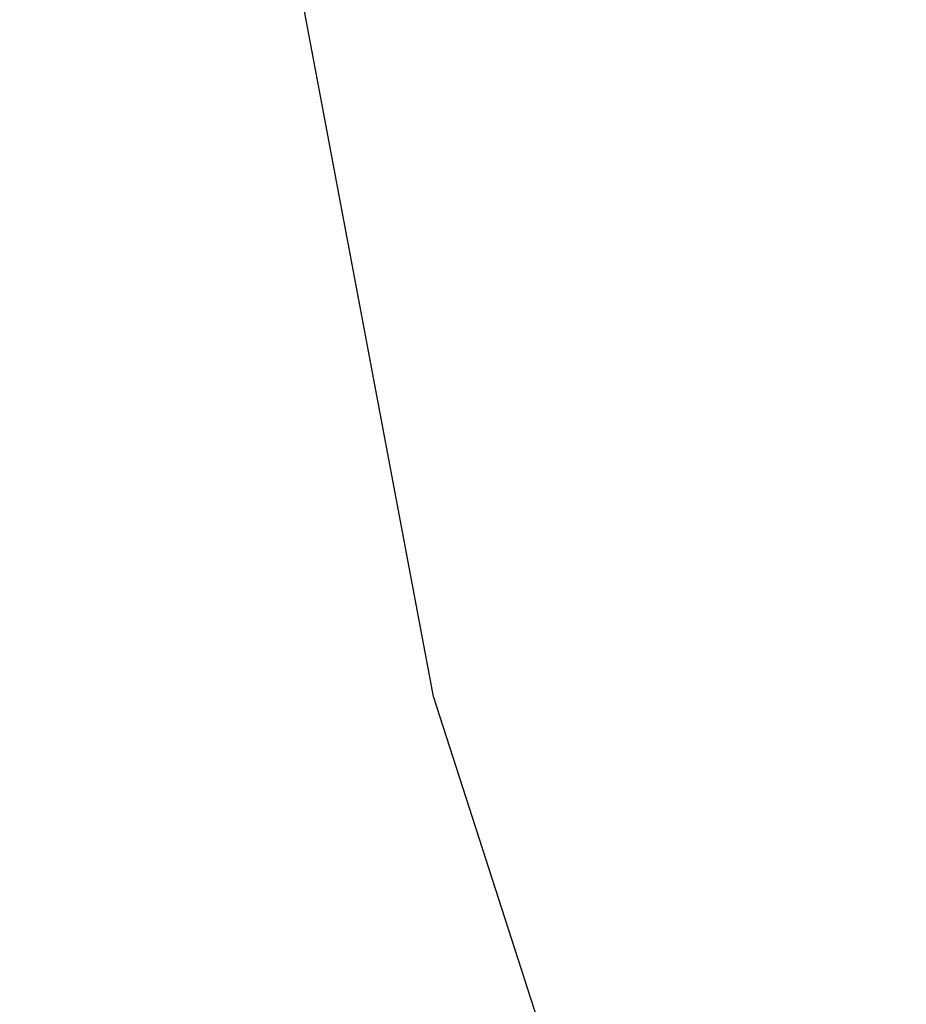
# Model space of a CAD drawing. Units: inches. Extents: x 3590 to 5167, y 65 to 1917.
# Tile 76 of 100: x 5045.839 to 5047.497, y 1787.19 to 1789.032. Entities that reach past the tile are written whole.
import ezdxf

# ---------------------------------------------------------------- set-up
doc = ezdxf.new("R2010")
doc.units = ezdxf.units.IN
for name, color, linetype, lineweight in [('A-ANNO-DIMS', 2, 'Continuous', 18), ('A-FLOR-PATT', 8, 'Continuous', 13), ('L-PLNT', 94, 'Continuous', 18)]:
    doc.layers.add(name, color=color, linetype=linetype, lineweight=lineweight)
doc.layers.add('DIENHOA', color=3, linetype='Continuous')
doc.styles.get("Standard").update_dxf_attribs({"font": 'arial.ttf'})
doc.dimstyles.new('ISO-25', dxfattribs={"dimtxt": 9, "dimasz": 2.5, "dimexe": 1.25, "dimexo": 0.625, "dimtad": 1, "dimdec": 1, "dimlunit": 3, "dimtxsty": 'Standard', "dimcen": 2.5, "dimadec": 0, "dimazin": 0, "dimtfac": 1, "dimtdec": 1, "dimtmove": 0, "dimatfit": 3, "dimfxl": 1, "dimarcsym": 0})

# ---------------------------------------------------------------- blocks, each defined once
blk = doc.blocks.new('Cay03_mb')
at = {"layer": 'DIENHOA'}
blk.add_lwpolyline([(23.687, -5.439), (-41, 82.202), (-91.832, 167.077), (-129.715, 249.451), (-155.553, 329.591), (-170.25, 407.762), (-174.71, 484.231), (-169.839, 559.263), (-156.54, 633.124)], dxfattribs=at)
blk = doc.blocks.new('*D322')
at = {"layer": 'A-ANNO-DIMS', "color": 0, "lineweight": -2, "transparency": 16777216}
for p, q in [((5035.7437, 1766.1842), (5035.7437, 1761.199)), ((5064.812, 1766.1842), (5064.812, 1761.199)), ((5038.2437, 1762.449), (5062.312, 1762.449)), ((5064.812, 1762.449), (5166.9911, 1762.449))]:
    blk.add_line(p, q, dxfattribs=at)
at = {"layer": 'A-ANNO-DIMS', "color": 0, "transparency": 16777216}
for points in [[(5038.2437, 1762.8657), (5038.2437, 1762.0323), (5035.7437, 1762.449)], [(5062.312, 1762.8657), (5062.312, 1762.0323), (5064.812, 1762.449)]]:
    blk.add_solid(points, dxfattribs=at)
at = {"layer": 'Defpoints', "color": 0, "transparency": 16777216}
for p in [(5035.7437, 1766.8092), (5064.812, 1766.8092), (5064.812, 1762.449)]:
    blk.add_point(p, dxfattribs=at)
at = {"layer": 'A-ANNO-DIMS', "color": 0, "transparency": 16777216, "insert": (5117.1516, 1767.6692), "char_height": 9, "attachment_point": 5}
blk.add_mtext('PLANT 2\'-5" TYP.', dxfattribs=at)

msp = doc.modelspace()

# ---------------------------------------------------------------- hatches: boundary and pattern name
at = {"layer": 'A-FLOR-PATT', "transparency": 33554687}
h = msp.add_hatch(dxfattribs=at)
h.set_pattern_fill('AR-HBONE', color=256, scale=0.2)
h.set_pattern_definition([(45, (-588.972, 0), (0, 28.73682), [60.96, -20.32]), (135, (-574.604, 14.368), (3e-15, 28.73682), [60.96, -20.32])])
h.paths.add_polyline_path([(5071.274, 1796.999), (4933.274, 1796.999), (4933.274, 1753.999), (4962.774, 1753.999, -0.414214), (4928.774, 1719.999), (4933.274, 1718.999), (4933.274, 1334.999), (5071.274, 1334.999)])
h.paths.add_polyline_path([(4951.78, 1521.0767), (4951.7151, 1521.0404), (4951.5634, 1520.8953)], flags=16)
h.paths.add_polyline_path([(4952.267, 1521.3764), (4952.1977, 1521.3711), (4952.1982, 1521.3556)], flags=0)
h.paths.add_polyline_path([(4967.0508, 1529.7283), (4965.2312, 1528.6944), (4963.4111, 1527.714), (4961.7565, 1526.8508), (4963.5889, 1527.4494), (4964.0356, 1527.478), (4962.9755, 1527.249), (4961.7602, 1526.852), (4959.7922, 1525.8341), (4958.005, 1524.8948), (4956.2403, 1523.9296), (4954.5039, 1522.9185), (4954.1294, 1522.6816), (4953.3605, 1521.9969), (4953.3656, 1521.9975), (4953.605, 1522.0637), (4955.1061, 1522.7608), (4956.9211, 1523.4341), (4958.6778, 1523.9151), (4960.3583, 1524.2004), (4961.9446, 1524.2861), (4964.1714, 1524.1085), (4965.9575, 1523.309), (4963.8627, 1522.9756), (4965.1874, 1522.499), (4963.3661, 1522.4971), (4961.5453, 1522.4868), (4959.7636, 1522.4608), (4958.3041, 1522.4188), (4957.9736, 1522.3883), (4956.3069, 1522.2324), (4954.7182, 1522.0714), (4953.2508, 1521.8992), (4953.5251, 1521.6228), (4954.3309, 1521.3788), (4956.2426, 1521.2299), (4958.0391, 1520.9295), (4959.6842, 1520.4834), (4961.1601, 1519.8957), (4963.107, 1518.8002), (4964.3929, 1517.3252), (4962.9731, 1517.726), (4964.5584, 1516.6606), (4965.4066, 1515.7078), (4963.5073, 1516.3218), (4961.68, 1517.0051), (4959.9348, 1517.7449), (4958.2821, 1518.5283), (4956.7322, 1519.3426), (4955.2953, 1520.1748), (4954.6715, 1520.5724), (4954.5128, 1520.6271), (4955.6585, 1519.3184), (4956.7026, 1517.9823), (4957.644, 1516.6466), (4958.4855, 1515.3344), (4959.55, 1513.524), (4960.4377, 1511.7694), (4958.8411, 1513.6196), (4957.4517, 1515.3249), (4955.8186, 1517.4586), (4956.6654, 1515.4476), (4957.1111, 1513.9229), (4957.4468, 1511.7143), (4957.0764, 1509.7929), (4956.5376, 1511.1103), (4955.9923, 1512.5689), (4955.4445, 1514.1251), (4954.8979, 1515.7352), (4954.3565, 1517.3555), (4953.8241, 1518.9425), (4953.3046, 1520.4525), (4953.0645, 1521.1156), (4952.9714, 1521.1461), (4952.9493, 1521.0865), (4952.7298, 1520.199), (4953.3698, 1518.0236), (4953.7571, 1516.3728), (4954.0512, 1514.7654), (4954.2645, 1513.2212), (4954.4712, 1511.1312), (4954.4971, 1510.4017), (4954.409, 1511.7601), (4954.2645, 1513.2212), (4954.0512, 1514.7654), (4953.7571, 1516.3728), (4953.3698, 1518.0236), (4952.8772, 1519.6981), (4952.7161, 1520.1412), (4952.533, 1519.0587), (4952.3743, 1517.7888), (4952.2192, 1516.3117), (4952.046, 1514.5999), (4951.8325, 1512.626), (4951.557, 1510.3626), (4951.2033, 1512.1682), (4950.8517, 1514.3393), (4950.9853, 1516.3759), (4951.6596, 1518.2862), (4952.5926, 1520.4808), (4952.3566, 1521.1299), (4951.855, 1520.3275), (4950.839, 1518.9083), (4949.7767, 1517.5866), (4948.9155, 1516.6173), (4948.111, 1515.2561), (4947.0891, 1513.5539), (4945.8894, 1511.6149), (4946.3259, 1513.4023), (4946.5624, 1514.2491), (4945.5277, 1513.3267), (4944.5811, 1512.5313), (4946.0177, 1514.5082), (4947.2044, 1516.0476), (4947.8933, 1517.3133), (4949.3069, 1518.7645), (4950.4142, 1519.7672), (4950.4513, 1519.8063), (4952.267, 1521.3764), (4951.6446, 1521.4932), (4950.4037, 1521.1795), (4948.0445, 1520.3587), (4946.1186, 1519.452), (4944.5718, 1518.4748), (4943.3496, 1517.4427), (4941.997, 1515.9197), (4941.6615, 1515.2748), (4942.8133, 1516.9897), (4944.5718, 1518.4748), (4946.1186, 1519.452), (4948.0445, 1520.3587), (4950.4037, 1521.1795), (4951.6446, 1521.4932), (4949.6468, 1521.8678), (4948.5998, 1521.7563), (4947.1263, 1521.5699), (4945.4202, 1521.3476), (4943.4497, 1521.1046), (4941.1832, 1520.856), (4942.8603, 1521.6126), (4943.8731, 1522.0301), (4942.9522, 1521.9093), (4941.4097, 1521.4851), (4939.5429, 1520.6702), (4938.9677, 1520.2255), (4940.7328, 1521.299), (4942.9522, 1521.9093), (4943.7018, 1522.0077), (4945.8942, 1522.7), (4947.5649, 1522.714), (4948.9209, 1522.5657), (4951.1314, 1522.1827), (4950.9706, 1522.2969), (4948.1292, 1523.0056), (4946.035, 1523.7067), (4944.2323, 1524.5214), (4942.7069, 1525.4611), (4941.4442, 1526.5371), (4940.4297, 1527.7606), (4939.6489, 1529.1431), (4941.4209, 1528.1223), (4943.1474, 1527.1325), (4944.8409, 1526.1746), (4946.5139, 1525.2496), (4948.1789, 1524.3586), (4948.3646, 1524.2634), (4946.4753, 1526.0446), (4945.1808, 1527.5404), (4944.1904, 1529.0334), (4943.4956, 1530.5398), (4943.2781, 1531.3597), (4942.4985, 1531.919), (4943.1135, 1531.7625), (4942.9593, 1533.6586), (4944.1395, 1531.9886), (4944.6117, 1531.3234), (4946.2016, 1530.4634), (4947.4857, 1529.5093), (4948.7903, 1528.2265), (4950.3675, 1526.2375), (4949.4855, 1528.1555), (4948.8513, 1530.1225), (4948.4905, 1532.0413), (4948.3811, 1533.9182), (4948.5006, 1535.7599), (4948.827, 1537.5728), (4949.418, 1535.5653), (4949.9568, 1533.5693), (4950.4641, 1531.5861), (4950.9606, 1529.6167), (4951.3911, 1527.9545), (4951.7235, 1530.6869), (4952.2011, 1532.5799), (4952.8891, 1534.3296), (4953.7703, 1535.9512), (4954.8273, 1537.46), (4954.5214, 1535.3897), (4954.2731, 1533.9368), (4955.58, 1535.6627), (4956.7476, 1536.7386), (4956.1585, 1534.7803), (4955.5892, 1532.8733), (4955.0434, 1531.0058), (4954.5249, 1529.1658), (4954.0377, 1527.3413), (4953.6383, 1525.733), (4953.6114, 1525.5856), (4953.3981, 1524.1657), (4953.3822, 1524.0089), (4954.0696, 1525.4756), (4954.9121, 1527.0217), (4956.1363, 1528.8935), (4957.8467, 1530.577), (4959.376, 1531.5401), (4958.256, 1530.104), (4957.1428, 1528.6629), (4956.0663, 1527.2431), (4955.0558, 1525.8705), (4954.141, 1524.5715), (4953.3516, 1523.372), (4953.3108, 1523.303), (4953.2725, 1522.9248), (4953.261, 1522.3821), (4954.1031, 1523.3727), (4954.63, 1524.2838), (4955.9615, 1526.3577), (4957.23, 1528.1297), (4958.4206, 1529.6086), (4960.0367, 1531.3679), (4961.3736, 1532.3752), (4962.1015, 1532.77), (4961.0699, 1531.0611), (4959.9873, 1529.4381), (4958.8685, 1527.908), (4958.1505, 1527.0074), (4959.8029, 1528.0031), (4961.5885, 1528.7926), (4963.3909, 1529.3278), (4965.2112, 1529.6321)], flags=16)
h.paths.add_polyline_path([(4962.9439, 1523.1819), (4961.1071, 1523.4219), (4960.3921, 1523.3616), (4962.3496, 1523.3306)], flags=0)
h.paths.add_polyline_path([(5049.5413, 1584.5509), (5049.4764, 1584.5146), (5049.3247, 1584.3695)], flags=16)
h.paths.add_polyline_path([(5050.0283, 1584.8506), (5049.959, 1584.8453), (5049.9595, 1584.8298)], flags=0)
h.paths.add_polyline_path([(5042.3331, 1581.949), (5043.8799, 1582.9262), (5045.8057, 1583.8329), (5048.165, 1584.6537), (5049.4058, 1584.9674), (5047.408, 1585.342), (5046.3611, 1585.2305), (5044.8876, 1585.0441), (5043.1814, 1584.8218), (5041.211, 1584.5788), (5038.9445, 1584.3301), (5040.6215, 1585.0868), (5041.6343, 1585.5043), (5040.7134, 1585.3835), (5039.1709, 1584.9593), (5037.3041, 1584.1444), (5036.729, 1583.6997), (5038.4941, 1584.7732), (5040.7134, 1585.3835), (5041.4631, 1585.4819), (5043.6555, 1586.1742), (5045.3261, 1586.1882), (5046.6821, 1586.0399), (5048.8927, 1585.6569), (5048.7319, 1585.7711), (5045.8905, 1586.4798), (5043.7962, 1587.1809), (5041.9936, 1587.9956), (5040.4682, 1588.9353), (5039.2055, 1590.0113), (5038.1909, 1591.2348), (5037.4102, 1592.6172), (5039.1822, 1591.5965), (5040.9087, 1590.6067), (5042.6022, 1589.6488), (5044.2752, 1588.7238), (5045.9402, 1587.8327), (5046.1258, 1587.7375), (5044.2366, 1589.5188), (5042.9421, 1591.0146), (5041.9517, 1592.5076), (5041.2569, 1594.014), (5041.0393, 1594.8339), (5040.2598, 1595.3932), (5040.8748, 1595.2367), (5040.7205, 1597.1328), (5041.9008, 1595.4628), (5042.373, 1594.7976), (5043.9629, 1593.9376), (5045.2469, 1592.9834), (5046.5515, 1591.7007), (5048.1288, 1589.7116), (5047.2467, 1591.6297), (5046.6125, 1593.5967), (5046.2518, 1595.5155), (5046.1423, 1597.3924), (5046.2619, 1599.2341), (5046.5883, 1601.047), (5047.1793, 1599.0394), (5047.7181, 1597.0435), (5048.2254, 1595.0603), (5048.7218, 1593.0909), (5049.1524, 1591.4287), (5049.4848, 1594.1611), (5049.9623, 1596.0541), (5050.6504, 1597.8038), (5051.5316, 1599.4254), (5052.5885, 1600.9341), (5052.2827, 1598.8638), (5052.0344, 1597.411), (5053.3413, 1599.1369), (5054.5088, 1600.2128), (5053.9198, 1598.2545), (5053.3504, 1596.3475), (5052.8046, 1594.48), (5052.2862, 1592.6399), (5051.799, 1590.8155), (5051.3996, 1589.2072), (5051.3727, 1589.0598), (5051.1593, 1587.6398), (5051.1435, 1587.4831), (5051.8308, 1588.9498), (5052.6734, 1590.4959), (5053.8975, 1592.3677), (5055.6079, 1594.0512), (5057.1373, 1595.0143), (5056.0172, 1593.5782), (5054.9041, 1592.1371), (5053.8275, 1590.7172), (5052.8171, 1589.3447), (5051.9023, 1588.0457), (5051.1129, 1586.8462), (5051.0721, 1586.7772), (5051.0338, 1586.399), (5051.0223, 1585.8563), (5051.8644, 1586.8469), (5052.3913, 1587.7579), (5053.7228, 1589.8318), (5054.9913, 1591.6039), (5056.1818, 1593.0828), (5057.798, 1594.8421), (5059.1349, 1595.8494), (5059.8628, 1596.2442), (5058.8312, 1594.5353), (5057.7486, 1592.9123), (5056.6298, 1591.3822), (5055.9117, 1590.4816), (5057.5642, 1591.4773), (5059.3498, 1592.2667), (5061.1521, 1592.802), (5062.9724, 1593.1062), (5064.812, 1593.2025), (5062.9925, 1592.1686), (5061.1724, 1591.1882), (5059.5178, 1590.325), (5061.3501, 1590.9236), (5061.7968, 1590.9522), (5060.7368, 1590.7232), (5059.5215, 1590.3262), (5057.5535, 1589.3082), (5055.7662, 1588.369), (5054.0016, 1587.4038), (5052.2652, 1586.3927), (5051.8907, 1586.1558), (5051.1218, 1585.4711), (5051.1268, 1585.4717), (5051.3663, 1585.5379), (5052.8673, 1586.235), (5054.6823, 1586.9082), (5056.4391, 1587.3893), (5058.1196, 1587.6745), (5059.7058, 1587.7602), (5061.9327, 1587.5827), (5063.7188, 1586.7832), (5061.624, 1586.4498), (5062.9487, 1585.9732), (5061.1274, 1585.9713), (5059.3065, 1585.961), (5057.5249, 1585.935), (5056.0654, 1585.893), (5055.7348, 1585.8625), (5054.0682, 1585.7066), (5052.4795, 1585.5456), (5051.012, 1585.3733), (5051.2864, 1585.097), (5052.0921, 1584.853), (5054.0039, 1584.7041), (5055.8004, 1584.4037), (5057.4455, 1583.9576), (5058.9213, 1583.3699), (5060.8683, 1582.2744), (5062.1541, 1580.7994), (5060.7343, 1581.2001), (5062.3197, 1580.1348), (5063.1679, 1579.182), (5061.2686, 1579.796), (5059.4412, 1580.4793), (5057.696, 1581.2191), (5056.0434, 1582.0025), (5054.4934, 1582.8168), (5053.0565, 1583.649), (5052.4328, 1584.0466), (5052.2741, 1584.1013), (5053.4197, 1582.7925), (5054.4639, 1581.4565), (5055.4053, 1580.1208), (5056.2467, 1578.8086), (5057.3112, 1576.9982), (5058.1989, 1575.2435), (5056.6023, 1577.0938), (5055.213, 1578.7991), (5053.5799, 1580.9327), (5054.4266, 1578.9218), (5054.8724, 1577.3971), (5055.2081, 1575.1885), (5054.8377, 1573.2671), (5054.2988, 1574.5845), (5053.7536, 1576.0431), (5053.2057, 1577.5993), (5052.6592, 1579.2094), (5052.1178, 1580.8297), (5051.5854, 1582.4167), (5051.0658, 1583.9267), (5050.8258, 1584.5898), (5050.7327, 1584.6203), (5050.7106, 1584.5606), (5050.4911, 1583.6732), (5051.1311, 1581.4978), (5051.5183, 1579.847), (5051.8125, 1578.2396), (5052.0257, 1576.6954), (5052.2325, 1574.6054), (5052.2584, 1573.8759), (5052.1703, 1575.2342), (5052.0257, 1576.6954), (5051.8125, 1578.2396), (5051.5183, 1579.847), (5051.1311, 1581.4978), (5050.6384, 1583.1723), (5050.4774, 1583.6154), (5050.2943, 1582.5329), (5050.1355, 1581.263), (5049.9805, 1579.7859), (5049.8072, 1578.074), (5049.5938, 1576.1002), (5049.3182, 1573.8368), (5048.9646, 1575.6424), (5048.6129, 1577.8135), (5048.7466, 1579.8501), (5049.4209, 1581.7604), (5050.3539, 1583.955), (5050.1179, 1584.6041), (5049.6163, 1583.8017), (5048.6003, 1582.3825), (5047.538, 1581.0608), (5046.6768, 1580.0915), (5045.8722, 1578.7303), (5044.8504, 1577.0281), (5043.6506, 1575.0891), (5044.0871, 1576.8765), (5044.3237, 1577.7233), (5043.289, 1576.8009), (5042.3423, 1576.0054), (5043.779, 1577.9824), (5044.9657, 1579.5218), (5045.6546, 1580.7875), (5047.0681, 1582.2386), (5048.1754, 1583.2413), (5048.2126, 1583.2805), (5050.0283, 1584.8506), (5049.4058, 1584.9674), (5048.165, 1584.6537), (5045.8057, 1583.8329), (5043.8799, 1582.9262), (5042.3331, 1581.949), (5041.1109, 1580.9168), (5039.7582, 1579.3939), (5039.4227, 1578.7489), (5040.5746, 1580.4639)], flags=16)
h.paths.add_polyline_path([(4954.7987, 1533.1203), (4954.2625, 1532.0793), (4953.8311, 1530.9346), (4953.5047, 1529.636), (4953.2834, 1528.1333), (4953.1672, 1526.3764), (4953.1563, 1524.315), (4953.2767, 1521.2363), (4952.8017, 1521.8418), (4951.557, 1521.9979), (4950.9758, 1521.9613), (4952.6606, 1521.941), (4952.8017, 1521.8418), (4953.1525, 1523.5926), (4953.1672, 1526.3764), (4953.2834, 1528.1333), (4953.6093, 1530.346), (4954.4556, 1532.5917)], flags=0)
h.paths.add_polyline_path([(5050.5629, 1585.316), (5049.3182, 1585.4721), (5048.737, 1585.4355), (5050.4219, 1585.4152), (5050.5629, 1585.316), (5050.9138, 1587.0668), (5050.9285, 1589.8506), (5051.0446, 1591.6075), (5051.3706, 1593.8202), (5052.2168, 1596.0659), (5052.56, 1596.5945), (5052.0238, 1595.5535), (5051.5924, 1594.4088), (5051.266, 1593.1102), (5051.0446, 1591.6075), (5050.9285, 1589.8506), (5050.9176, 1587.7892), (5051.038, 1584.7105)], flags=0)
h.paths.add_polyline_path([(5058.1533, 1586.8358), (5060.1109, 1586.8048), (5060.7051, 1586.6561), (5058.8684, 1586.8961)], flags=0)
h.paths.add_polyline_path([(5049.5413, 1430.9361), (5049.4764, 1430.8998), (5049.3247, 1430.7547)], flags=16)
h.paths.add_polyline_path([(5050.0283, 1431.2359), (5049.959, 1431.2305), (5049.9595, 1431.215)], flags=0)
h.paths.add_polyline_path([(5046.5883, 1447.4322), (5047.1793, 1445.4247), (5047.7181, 1443.4287), (5048.2254, 1441.4455), (5048.7218, 1439.4761), (5049.1524, 1437.8139), (5049.4848, 1440.5463), (5049.9623, 1442.4393), (5050.6504, 1444.189), (5051.5316, 1445.8106), (5052.5885, 1447.3194), (5052.2827, 1445.2491), (5052.0344, 1443.7962), (5053.3413, 1445.5221), (5054.5088, 1446.598), (5053.9198, 1444.6397), (5053.3504, 1442.7327), (5052.8046, 1440.8652), (5052.2862, 1439.0252), (5051.799, 1437.2007), (5051.3996, 1435.5924), (5051.3727, 1435.445), (5051.1593, 1434.0251), (5051.1435, 1433.8683), (5051.8308, 1435.335), (5052.6734, 1436.8811), (5053.8975, 1438.7529), (5055.6079, 1440.4364), (5057.1373, 1441.3995), (5056.0172, 1439.9634), (5054.9041, 1438.5223), (5053.8275, 1437.1025), (5052.8171, 1435.7299), (5051.9023, 1434.4309), (5051.1129, 1433.2314), (5051.0721, 1433.1624), (5051.0338, 1432.7842), (5051.0223, 1432.2415), (5051.8644, 1433.2321), (5052.3913, 1434.1432), (5053.7228, 1436.2171), (5054.9913, 1437.9891), (5056.1818, 1439.468), (5057.798, 1441.2273), (5059.1349, 1442.2346), (5059.8628, 1442.6294), (5058.8312, 1440.9205), (5057.7486, 1439.2975), (5056.6298, 1437.7674), (5055.9117, 1436.8668), (5057.5642, 1437.8625), (5059.3498, 1438.652), (5061.1521, 1439.1872), (5062.9724, 1439.4915), (5064.812, 1439.5877), (5062.9925, 1438.5538), (5061.1724, 1437.5734), (5059.5178, 1436.7102), (5061.3501, 1437.3088), (5061.7968, 1437.3374), (5060.7368, 1437.1084), (5059.5215, 1436.7114), (5057.5535, 1435.6935), (5055.7662, 1434.7542), (5054.0016, 1433.789), (5052.2652, 1432.7779), (5051.8907, 1432.541), (5051.1218, 1431.8563), (5051.1268, 1431.8569), (5051.3663, 1431.9231), (5052.8673, 1432.6202), (5054.6823, 1433.2935), (5056.4391, 1433.7745), (5058.1196, 1434.0598), (5059.7058, 1434.1455), (5061.9327, 1433.9679), (5063.7188, 1433.1684), (5061.624, 1432.8351), (5062.9487, 1432.3584), (5061.1274, 1432.3566), (5059.3065, 1432.3462), (5057.5249, 1432.3202), (5056.0654, 1432.2782), (5055.7348, 1432.2477), (5054.0682, 1432.0918), (5052.4795, 1431.9308), (5051.012, 1431.7586), (5051.2864, 1431.4822), (5052.0921, 1431.2382), (5054.0039, 1431.0893), (5055.8004, 1430.7889), (5057.4455, 1430.3428), (5058.9213, 1429.7551), (5060.8683, 1428.6596), (5062.1541, 1427.1846), (5060.7343, 1427.5854), (5062.3197, 1426.52), (5063.1679, 1425.5672), (5061.2686, 1426.1812), (5059.4412, 1426.8645), (5057.696, 1427.6043), (5056.0434, 1428.3877), (5054.4934, 1429.202), (5053.0565, 1430.0342), (5052.4328, 1430.4318), (5052.2741, 1430.4865), (5053.4197, 1429.1778), (5054.4639, 1427.8417), (5055.4053, 1426.506), (5056.2467, 1425.1938), (5057.3112, 1423.3834), (5058.1989, 1421.6288), (5056.6023, 1423.479), (5055.213, 1425.1843), (5053.5799, 1427.318), (5054.4266, 1425.307), (5054.8724, 1423.7823), (5055.2081, 1421.5737), (5054.8377, 1419.6523), (5054.2988, 1420.9697), (5053.7536, 1422.4283), (5053.2057, 1423.9845), (5052.6592, 1425.5946), (5052.1178, 1427.2149), (5051.5854, 1428.8019), (5051.0658, 1430.3119), (5050.8258, 1430.975), (5050.7327, 1431.0055), (5050.7106, 1430.9459), (5050.4911, 1430.0585), (5051.1311, 1427.883), (5051.5183, 1426.2322), (5051.8125, 1424.6248), (5052.0257, 1423.0806), (5052.2325, 1420.9906), (5052.2584, 1420.2611), (5052.1703, 1421.6195), (5052.0257, 1423.0806), (5051.8125, 1424.6248), (5051.5183, 1426.2322), (5051.1311, 1427.883), (5050.6384, 1429.5575), (5050.4774, 1430.0006), (5050.2943, 1428.9181), (5050.1355, 1427.6482), (5049.9805, 1426.1711), (5049.8072, 1424.4593), (5049.5938, 1422.4854), (5049.3182, 1420.222), (5048.9646, 1422.0276), (5048.6129, 1424.1987), (5048.7466, 1426.2353), (5049.4209, 1428.1457), (5050.3539, 1430.3403), (5050.1179, 1430.9893), (5049.6163, 1430.1869), (5048.6003, 1428.7677), (5047.538, 1427.446), (5046.6768, 1426.4767), (5045.8722, 1425.1155), (5044.8504, 1423.4133), (5043.6506, 1421.4744), (5044.0871, 1423.2617), (5044.3237, 1424.1085), (5043.289, 1423.1861), (5042.3423, 1422.3907), (5043.779, 1424.3677), (5044.9657, 1425.907), (5045.6546, 1427.1727), (5047.0681, 1428.6239), (5048.1754, 1429.6266), (5048.2126, 1429.6657), (5050.0283, 1431.2359), (5049.4058, 1431.3526), (5048.165, 1431.0389), (5045.8057, 1430.2181), (5043.8799, 1429.3114), (5042.3331, 1428.3342), (5041.1109, 1427.3021), (5039.7582, 1425.7791), (5039.4227, 1425.1342), (5040.5746, 1426.8491), (5042.3331, 1428.3342), (5043.8799, 1429.3114), (5045.8057, 1430.2181), (5048.165, 1431.0389), (5049.4058, 1431.3526), (5047.408, 1431.7272), (5046.3611, 1431.6157), (5044.8876, 1431.4293), (5043.1814, 1431.207), (5041.211, 1430.964), (5038.9445, 1430.7154), (5040.6215, 1431.4721), (5041.6343, 1431.8895), (5040.7134, 1431.7687), (5039.1709, 1431.3445), (5037.3041, 1430.5296), (5036.729, 1430.0849), (5038.4941, 1431.1584), (5040.7134, 1431.7687), (5041.4631, 1431.8671), (5043.6555, 1432.5594), (5045.3261, 1432.5734), (5046.6821, 1432.4251), (5048.8927, 1432.0421), (5048.7319, 1432.1563), (5045.8905, 1432.865), (5043.7962, 1433.5661), (5041.9936, 1434.3808), (5040.4682, 1435.3205), (5039.2055, 1436.3965), (5038.1909, 1437.62), (5037.4102, 1439.0025), (5039.1822, 1437.9817), (5040.9087, 1436.9919), (5042.6022, 1436.034), (5044.2752, 1435.109), (5045.9402, 1434.218), (5046.1258, 1434.1228), (5044.2366, 1435.904), (5042.9421, 1437.3998), (5041.9517, 1438.8928), (5041.2569, 1440.3993), (5041.0393, 1441.2191), (5040.2598, 1441.7784), (5040.8748, 1441.6219), (5040.7205, 1443.518), (5041.9008, 1441.848), (5042.373, 1441.1828), (5043.9629, 1440.3228), (5045.2469, 1439.3687), (5046.5515, 1438.0859), (5048.1288, 1436.0969), (5047.2467, 1438.0149), (5046.6125, 1439.9819), (5046.2518, 1441.9007), (5046.1423, 1443.7776), (5046.2619, 1445.6193)], flags=16)
h.paths.add_polyline_path([(5052.3818, 1444.255), (5051.6226, 1442.7799), (5052.0238, 1441.9388), (5052.56, 1442.9797)], flags=0)
h.paths.add_polyline_path([(5050.5629, 1431.7012), (5049.3182, 1431.8573), (5048.737, 1431.8207), (5050.4219, 1431.8004)], flags=0)
h.paths.add_polyline_path([(5058.1533, 1433.221), (5060.1109, 1433.19), (5060.7051, 1433.0413), (5058.8684, 1433.2813)], flags=0)
h.paths.add_polyline_path([(5049.5413, 1352.2853), (5049.4764, 1352.249), (5049.3247, 1352.104)], flags=16)
h.paths.add_polyline_path([(5050.0283, 1352.5851), (5049.959, 1352.5797), (5049.9595, 1352.5642)], flags=0)
h.paths.add_polyline_path([(5046.5883, 1368.7815), (5047.1793, 1366.7739), (5047.7181, 1364.778), (5048.2254, 1362.7947), (5048.7218, 1360.8253), (5049.1524, 1359.1631), (5049.4848, 1361.8955), (5049.9623, 1363.7886), (5050.6504, 1365.5383), (5051.5316, 1367.1599), (5052.5885, 1368.6686), (5052.2827, 1366.5983), (5052.0344, 1365.1455), (5053.3413, 1366.8713), (5054.5088, 1367.9472), (5053.9198, 1365.9889), (5053.3504, 1364.082), (5052.8046, 1362.2144), (5052.2862, 1360.3744), (5051.799, 1358.5499), (5051.3996, 1356.9416), (5051.3727, 1356.7943), (5051.1593, 1355.3743), (5051.1435, 1355.2175), (5051.8308, 1356.6843), (5052.6734, 1358.2304), (5053.8975, 1360.1022), (5055.6079, 1361.7857), (5057.1373, 1362.7488), (5056.0172, 1361.3126), (5054.9041, 1359.8716), (5053.8275, 1358.4517), (5052.8171, 1357.0792), (5051.9023, 1355.7801), (5051.1129, 1354.5807), (5051.0721, 1354.5116), (5051.0338, 1354.1334), (5051.0223, 1353.5908), (5051.8644, 1354.5814), (5052.3913, 1355.4924), (5053.7228, 1357.5663), (5054.9913, 1359.3383), (5056.1818, 1360.8173), (5057.798, 1362.5766), (5059.1349, 1363.5838), (5059.8628, 1363.9786), (5058.8312, 1362.2698), (5057.7486, 1360.6468), (5056.6298, 1359.1167), (5055.9117, 1358.2161), (5057.5642, 1359.2118), (5059.3498, 1360.0012), (5061.1521, 1360.5365), (5062.9724, 1360.8407), (5064.812, 1360.937), (5062.9925, 1359.9031), (5061.1724, 1358.9227), (5059.5178, 1358.0595), (5061.3501, 1358.658), (5061.7968, 1358.6867), (5060.7368, 1358.4577), (5059.5215, 1358.0607), (5057.5535, 1357.0427), (5055.7662, 1356.1035), (5054.0016, 1355.1382), (5052.2652, 1354.1272), (5051.8907, 1353.8903), (5051.1218, 1353.2055), (5051.1268, 1353.2062), (5051.3663, 1353.2723), (5052.8673, 1353.9695), (5054.6823, 1354.6427), (5056.4391, 1355.1238), (5058.1196, 1355.409), (5059.7058, 1355.4947), (5061.9327, 1355.3171), (5063.7188, 1354.5177), (5061.624, 1354.1843), (5062.9487, 1353.7076), (5061.1274, 1353.7058), (5059.3065, 1353.6955), (5057.5249, 1353.6694), (5056.0654, 1353.6274), (5055.7348, 1353.5969), (5054.0682, 1353.441), (5052.4795, 1353.2801), (5051.012, 1353.1078), (5051.2864, 1352.8314), (5052.0921, 1352.5875), (5054.0039, 1352.4385), (5055.8004, 1352.1382), (5057.4455, 1351.692), (5058.9213, 1351.1043), (5060.8683, 1350.0089), (5062.1541, 1348.5338), (5060.7343, 1348.9346), (5062.3197, 1347.8692), (5063.1679, 1346.9164), (5061.2686, 1347.5304), (5059.4412, 1348.2137), (5057.696, 1348.9535), (5056.0434, 1349.737), (5054.4934, 1350.5512), (5053.0565, 1351.3834), (5052.4328, 1351.781), (5052.2741, 1351.8357), (5053.4197, 1350.527), (5054.4639, 1349.191), (5055.4053, 1347.8553), (5056.2467, 1346.543), (5057.3112, 1344.7326), (5058.1989, 1342.978), (5056.6023, 1344.8282), (5055.213, 1346.5335), (5053.5799, 1348.6672), (5054.4266, 1346.6563), (5054.8724, 1345.1316), (5055.2081, 1342.923), (5054.8377, 1341.0015), (5054.2988, 1342.3189), (5053.7536, 1343.7776), (5053.2057, 1345.3337), (5052.6592, 1346.9438), (5052.1178, 1348.5642), (5051.5854, 1350.1512), (5051.0658, 1351.6611), (5050.8258, 1352.3243), (5050.7327, 1352.3547), (5050.7106, 1352.2951), (5050.4911, 1351.4077), (5051.1311, 1349.2323), (5051.5183, 1347.5814), (5051.8125, 1345.974), (5052.0257, 1344.4298), (5052.2325, 1342.3399), (5052.2584, 1341.6104), (5052.1703, 1342.9687), (5052.0257, 1344.4298), (5051.8125, 1345.974), (5051.5183, 1347.5814), (5051.1311, 1349.2323), (5050.6384, 1350.9068), (5050.4774, 1351.3498), (5050.2943, 1350.2674), (5050.1355, 1348.9975), (5049.9805, 1347.5203), (5049.8072, 1345.8085), (5049.5938, 1343.8346), (5049.3182, 1341.5712), (5048.9646, 1343.3768), (5048.6129, 1345.548), (5048.7466, 1347.5846), (5049.4209, 1349.4949), (5050.3539, 1351.6895), (5050.1179, 1352.3385), (5049.6163, 1351.5362), (5048.6003, 1350.1169), (5047.538, 1348.7952), (5046.6768, 1347.826), (5045.8722, 1346.4647), (5044.8504, 1344.7625), (5043.6506, 1342.8236), (5044.0871, 1344.611), (5044.3237, 1345.4578), (5043.289, 1344.5353), (5042.3423, 1343.7399), (5043.779, 1345.7169), (5044.9657, 1347.2563), (5045.6546, 1348.522), (5047.0681, 1349.9731), (5048.1754, 1350.9758), (5048.2126, 1351.0149), (5050.0283, 1352.5851), (5049.4058, 1352.7018), (5048.165, 1352.3882), (5045.8057, 1351.5673), (5043.8799, 1350.6606), (5042.3331, 1349.6835), (5041.1109, 1348.6513), (5039.7582, 1347.1283), (5039.4227, 1346.4834), (5040.5746, 1348.1984), (5042.3331, 1349.6835), (5043.8799, 1350.6606), (5045.8057, 1351.5673), (5048.165, 1352.3882), (5049.4058, 1352.7018), (5047.408, 1353.0765), (5046.3611, 1352.965), (5044.8876, 1352.7785), (5043.1814, 1352.5563), (5041.211, 1352.3133), (5038.9445, 1352.0646), (5040.6215, 1352.8213), (5041.6343, 1353.2388), (5040.7134, 1353.1179), (5039.1709, 1352.6938), (5037.3041, 1351.8788), (5036.729, 1351.4341), (5038.4941, 1352.5076), (5040.7134, 1353.1179), (5041.4631, 1353.2163), (5043.6555, 1353.9086), (5045.3261, 1353.9226), (5046.6821, 1353.7744), (5048.8927, 1353.3914), (5048.7319, 1353.5055), (5045.8905, 1354.2143), (5043.7962, 1354.9153), (5041.9936, 1355.7301), (5040.4682, 1356.6698), (5039.2055, 1357.7457), (5038.1909, 1358.9693), (5037.4102, 1360.3517), (5039.1822, 1359.331), (5040.9087, 1358.3411), (5042.6022, 1357.3832), (5044.2752, 1356.4582), (5045.9402, 1355.5672), (5046.1258, 1355.472), (5044.2366, 1357.2532), (5042.9421, 1358.7491), (5041.9517, 1360.242), (5041.2569, 1361.7485), (5041.0393, 1362.5683), (5040.2598, 1363.1277), (5040.8748, 1362.9711), (5040.7205, 1364.8672), (5041.9008, 1363.1972), (5042.373, 1362.532), (5043.9629, 1361.6721), (5045.2469, 1360.7179), (5046.5515, 1359.4351), (5048.1288, 1357.4461), (5047.2467, 1359.3641), (5046.6125, 1361.3312), (5046.2518, 1363.2499), (5046.1423, 1365.1269), (5046.2619, 1366.9685)], flags=16)
h.paths.add_polyline_path([(5052.3818, 1365.6042), (5051.6226, 1364.1291), (5052.0238, 1363.288), (5052.56, 1364.3289)], flags=0)
h.paths.add_polyline_path([(4951.78, 1698.0408), (4951.7151, 1698.0045), (4951.5634, 1697.8594)], flags=16)
h.paths.add_polyline_path([(4952.267, 1698.3406), (4952.1977, 1698.3352), (4952.1982, 1698.3197)], flags=0)
h.paths.add_polyline_path([(4957.0764, 1686.757), (4956.5376, 1688.0744), (4955.9923, 1689.533), (4955.4445, 1691.0892), (4954.8979, 1692.6993), (4954.3565, 1694.3196), (4953.8241, 1695.9066), (4953.3046, 1697.4166), (4953.0645, 1698.0797), (4952.9714, 1698.1102), (4952.9493, 1698.0506), (4952.7298, 1697.1632), (4953.3698, 1694.9877), (4953.7571, 1693.3369), (4954.0512, 1691.7295), (4954.2645, 1690.1853), (4954.4712, 1688.0953), (4954.4971, 1687.3658), (4954.409, 1688.7242), (4954.2645, 1690.1853), (4954.0512, 1691.7295), (4953.7571, 1693.3369), (4953.3698, 1694.9877), (4952.8772, 1696.6622), (4952.7161, 1697.1053), (4952.533, 1696.0228), (4952.3743, 1694.7529), (4952.2192, 1693.2758), (4952.046, 1691.564), (4951.8325, 1689.5901), (4951.557, 1687.3267), (4951.2033, 1689.1323), (4950.8517, 1691.3034), (4950.9853, 1693.34), (4951.6596, 1695.2504), (4952.5926, 1697.445), (4952.3566, 1698.094), (4951.855, 1697.2916), (4950.839, 1695.8724), (4949.7767, 1694.5507), (4948.9155, 1693.5814), (4948.111, 1692.2202), (4947.0891, 1690.518), (4945.8894, 1688.5791), (4946.3259, 1690.3664), (4946.5624, 1691.2132), (4945.5277, 1690.2908), (4944.5811, 1689.4954), (4946.0177, 1691.4724), (4947.2044, 1693.0117), (4947.8933, 1694.2774), (4949.3069, 1695.7286), (4950.4142, 1696.7313), (4950.4513, 1696.7704), (4952.267, 1698.3406), (4951.6446, 1698.4573), (4950.4037, 1698.1436), (4948.0445, 1697.3228), (4946.1186, 1696.4161), (4944.5718, 1695.4389), (4943.3496, 1694.4068), (4941.997, 1692.8838), (4941.6615, 1692.2389), (4942.8133, 1693.9538), (4944.5718, 1695.4389), (4946.1186, 1696.4161), (4948.0445, 1697.3228), (4950.4037, 1698.1436), (4951.6446, 1698.4573), (4949.6468, 1698.8319), (4948.5998, 1698.7204), (4947.1263, 1698.534), (4945.4202, 1698.3117), (4943.4497, 1698.0687), (4941.1832, 1697.8201), (4942.8603, 1698.5768), (4943.8731, 1698.9942), (4942.9522, 1698.8734), (4941.4097, 1698.4492), (4939.5429, 1697.6343), (4938.9677, 1697.1896), (4940.7328, 1698.2631), (4942.9522, 1698.8734), (4943.7018, 1698.9718), (4945.8942, 1699.6641), (4947.5649, 1699.6781), (4948.9209, 1699.5298), (4951.1314, 1699.1468), (4950.9706, 1699.261), (4948.1292, 1699.9697), (4946.035, 1700.6708), (4944.2323, 1701.4855), (4942.7069, 1702.4252), (4941.4442, 1703.5012), (4940.4297, 1704.7247), (4939.6489, 1706.1072), (4941.4209, 1705.0864), (4943.1474, 1704.0966), (4944.8409, 1703.1387), (4946.5139, 1702.2137), (4948.1789, 1701.3227), (4948.3646, 1701.2275), (4946.4753, 1703.0087), (4945.1808, 1704.5045), (4944.1904, 1705.9975), (4943.4956, 1707.504), (4943.2781, 1708.3238), (4942.4985, 1708.8831), (4943.1135, 1708.7266), (4942.9593, 1710.6227), (4944.1395, 1708.9527), (4944.6117, 1708.2875), (4946.2016, 1707.4275), (4947.4857, 1706.4734), (4948.7903, 1705.1906), (4950.3675, 1703.2016), (4949.4855, 1705.1196), (4948.8513, 1707.0866), (4948.4905, 1709.0054), (4948.3811, 1710.8823), (4948.5006, 1712.724), (4948.827, 1714.5369), (4949.418, 1712.5294), (4949.9568, 1710.5334), (4950.4641, 1708.5502), (4950.9606, 1706.5808), (4951.3911, 1704.9186), (4951.7235, 1707.651), (4952.2011, 1709.544), (4952.8891, 1711.2937), (4953.7703, 1712.9153), (4954.8273, 1714.4241), (4954.5214, 1712.3538), (4954.2731, 1710.9009), (4955.58, 1712.6268), (4956.7476, 1713.7027), (4956.1585, 1711.7444), (4955.5892, 1709.8374), (4955.0434, 1707.9699), (4954.5249, 1706.1299), (4954.0377, 1704.3054), (4953.6383, 1702.6971), (4953.6114, 1702.5497), (4953.3981, 1701.1298), (4953.3822, 1700.973), (4954.0696, 1702.4397), (4954.9121, 1703.9858), (4956.1363, 1705.8576), (4957.8467, 1707.5411), (4959.376, 1708.5042), (4958.256, 1707.0681), (4957.1428, 1705.627), (4956.0663, 1704.2072), (4955.0558, 1702.8346), (4954.141, 1701.5356), (4953.3516, 1700.3361), (4953.3108, 1700.2671), (4953.2725, 1699.8889), (4953.261, 1699.3462), (4954.1031, 1700.3368), (4954.63, 1701.2479), (4955.9615, 1703.3218), (4957.23, 1705.0938), (4958.4206, 1706.5727), (4960.0367, 1708.332), (4961.3736, 1709.3393), (4962.1015, 1709.7341), (4961.0699, 1708.0252), (4959.9873, 1706.4022), (4958.8685, 1704.8721), (4958.1505, 1703.9715), (4959.8029, 1704.9672), (4961.5885, 1705.7567), (4963.3909, 1706.2919), (4965.2112, 1706.5962), (4967.0508, 1706.6924), (4965.2312, 1705.6585), (4963.4111, 1704.6781), (4961.7565, 1703.8149), (4963.5889, 1704.4135), (4964.0356, 1704.4421), (4962.9755, 1704.2131), (4961.7602, 1703.8161), (4959.7922, 1702.7982), (4958.005, 1701.8589), (4956.2403, 1700.8937), (4954.5039, 1699.8826), (4954.1294, 1699.6457), (4953.3605, 1698.961), (4953.3656, 1698.9616), (4953.605, 1699.0278), (4955.1061, 1699.7249), (4956.9211, 1700.3982), (4958.6778, 1700.8792), (4960.3583, 1701.1645), (4961.9446, 1701.2502), (4964.1714, 1701.0726), (4965.9575, 1700.2731), (4963.8627, 1699.9398), (4965.1874, 1699.4631), (4963.3661, 1699.4613), (4961.5453, 1699.4509), (4959.7636, 1699.4249), (4958.3041, 1699.3829), (4957.9736, 1699.3524), (4956.3069, 1699.1965), (4954.7182, 1699.0355), (4953.2508, 1698.8633), (4953.5251, 1698.5869), (4954.3309, 1698.3429), (4956.2426, 1698.194), (4958.0391, 1697.8936), (4959.6842, 1697.4475), (4961.1601, 1696.8598), (4963.107, 1695.7643), (4964.3929, 1694.2893), (4962.9731, 1694.6901), (4964.5584, 1693.6247), (4965.4066, 1692.6719), (4963.5073, 1693.2859), (4961.68, 1693.9692), (4959.9348, 1694.709), (4958.2821, 1695.4924), (4956.7322, 1696.3067), (4955.2953, 1697.1389), (4954.6715, 1697.5365), (4954.5128, 1697.5912), (4955.6585, 1696.2825), (4956.7026, 1694.9464), (4957.644, 1693.6107), (4958.4855, 1692.2985), (4959.55, 1690.4881), (4960.4377, 1688.7335), (4958.8411, 1690.5837), (4957.4517, 1692.289), (4955.8186, 1694.4227), (4956.6654, 1692.4117), (4957.1111, 1690.887), (4957.4468, 1688.6784)], flags=16)
h.paths.add_polyline_path([(5050.5629, 1353.0504), (5049.3182, 1353.2065), (5048.737, 1353.1699), (5050.4219, 1353.1496)], flags=0)
h.paths.add_polyline_path([(4951.78, 1351.4861), (4951.7151, 1351.4498), (4951.5634, 1351.3047)], flags=16)
h.paths.add_polyline_path([(4952.267, 1351.7858), (4952.1977, 1351.7805), (4952.1982, 1351.765)], flags=0)
h.paths.add_polyline_path([(4954.8273, 1367.8693), (4954.5214, 1365.799), (4954.2731, 1364.3462), (4955.58, 1366.0721), (4956.7476, 1367.148), (4956.1585, 1365.1897), (4955.5892, 1363.2827), (4955.0434, 1361.4152), (4954.5249, 1359.5752), (4954.0377, 1357.7507), (4953.6383, 1356.1424), (4953.6114, 1355.995), (4953.3981, 1354.575), (4953.3822, 1354.4183), (4954.0696, 1355.885), (4954.9121, 1357.4311), (4956.1363, 1359.3029), (4957.8467, 1360.9864), (4959.376, 1361.9495), (4958.256, 1360.5134), (4957.1428, 1359.0723), (4956.0663, 1357.6524), (4955.0558, 1356.2799), (4954.141, 1354.9809), (4953.3516, 1353.7814), (4953.3108, 1353.7124), (4953.2725, 1353.3342), (4953.261, 1352.7915), (4954.1031, 1353.7821), (4954.63, 1354.6931), (4955.9615, 1356.7671), (4957.23, 1358.5391), (4958.4206, 1360.018), (4960.0367, 1361.7773), (4961.3736, 1362.7846), (4962.1015, 1363.1794), (4961.0699, 1361.4705), (4959.9873, 1359.8475), (4958.8685, 1358.3174), (4958.1505, 1357.4168), (4959.8029, 1358.4125), (4961.5885, 1359.202), (4963.3909, 1359.7372), (4965.2112, 1360.0414), (4967.0508, 1360.1377), (4965.2312, 1359.1038), (4963.4111, 1358.1234), (4961.7565, 1357.2602), (4963.5889, 1357.8588), (4964.0356, 1357.8874), (4962.9755, 1357.6584), (4961.7602, 1357.2614), (4959.7922, 1356.2435), (4958.005, 1355.3042), (4956.2403, 1354.339), (4954.5039, 1353.3279), (4954.1294, 1353.091), (4953.3605, 1352.4063), (4953.3656, 1352.4069), (4953.605, 1352.4731), (4955.1061, 1353.1702), (4956.9211, 1353.8434), (4958.6778, 1354.3245), (4960.3583, 1354.6098), (4961.9446, 1354.6954), (4964.1714, 1354.5179), (4965.9575, 1353.7184), (4963.8627, 1353.385), (4965.1874, 1352.9084), (4963.3661, 1352.9065), (4961.5453, 1352.8962), (4959.7636, 1352.8702), (4958.3041, 1352.8282), (4957.9736, 1352.7977), (4956.3069, 1352.6418), (4954.7182, 1352.4808), (4953.2508, 1352.3085), (4953.5251, 1352.0322), (4954.3309, 1351.7882), (4956.2426, 1351.6393), (4958.0391, 1351.3389), (4959.6842, 1350.8928), (4961.1601, 1350.3051), (4963.107, 1349.2096), (4964.3929, 1347.7346), (4962.9731, 1348.1354), (4964.5584, 1347.07), (4965.4066, 1346.1172), (4963.5073, 1346.7312), (4961.68, 1347.4145), (4959.9348, 1348.1543), (4958.2821, 1348.9377), (4956.7322, 1349.752), (4955.2953, 1350.5842), (4954.6715, 1350.9818), (4954.5128, 1351.0365), (4955.6585, 1349.7278), (4956.7026, 1348.3917), (4957.644, 1347.056), (4958.4855, 1345.7438), (4959.55, 1343.9334), (4960.4377, 1342.1788), (4958.8411, 1344.029), (4957.4517, 1345.7343), (4955.8186, 1347.8679), (4956.6654, 1345.857), (4957.1111, 1344.3323), (4957.4468, 1342.1237), (4957.0764, 1340.2023), (4956.5376, 1341.5197), (4955.9923, 1342.9783), (4955.4445, 1344.5345), (4954.8979, 1346.1446), (4954.3565, 1347.7649), (4953.8241, 1349.3519), (4953.3046, 1350.8619), (4953.0645, 1351.525), (4952.9714, 1351.5555), (4952.9493, 1351.4959), (4952.7298, 1350.6084), (4953.3698, 1348.433), (4953.7571, 1346.7822), (4954.0512, 1345.1748), (4954.2645, 1343.6306), (4954.4712, 1341.5406), (4954.4971, 1340.8111), (4954.409, 1342.1695), (4954.2645, 1343.6306), (4954.0512, 1345.1748), (4953.7571, 1346.7822), (4953.3698, 1348.433), (4952.8772, 1350.1075), (4952.7161, 1350.5506), (4952.533, 1349.4681), (4952.3743, 1348.1982), (4952.2192, 1346.7211), (4952.046, 1345.0093), (4951.8325, 1343.0354), (4951.557, 1340.772), (4951.2033, 1342.5776), (4950.8517, 1344.7487), (4950.9853, 1346.7853), (4951.6596, 1348.6956), (4952.5926, 1350.8902), (4952.3566, 1351.5393), (4951.855, 1350.7369), (4950.839, 1349.3177), (4949.7767, 1347.996), (4948.9155, 1347.0267), (4948.111, 1345.6655), (4947.0891, 1343.9633), (4945.8894, 1342.0243), (4946.3259, 1343.8117), (4946.5624, 1344.6585), (4945.5277, 1343.7361), (4944.5811, 1342.9407), (4946.0177, 1344.9176), (4947.2044, 1346.457), (4947.8933, 1347.7227), (4949.3069, 1349.1739), (4950.4142, 1350.1766), (4950.4513, 1350.2157), (4952.267, 1351.7858), (4951.6446, 1351.9026), (4950.4037, 1351.5889), (4948.0445, 1350.7681), (4946.1186, 1349.8614), (4944.5718, 1348.8842), (4943.3496, 1347.852), (4941.997, 1346.3291), (4941.6615, 1345.6841), (4942.8133, 1347.3991), (4944.5718, 1348.8842), (4946.1186, 1349.8614), (4948.0445, 1350.7681), (4950.4037, 1351.5889), (4951.6446, 1351.9026), (4949.6468, 1352.2772), (4948.5998, 1352.1657), (4947.1263, 1351.9793), (4945.4202, 1351.757), (4943.4497, 1351.514), (4941.1832, 1351.2653), (4942.8603, 1352.022), (4943.8731, 1352.4395), (4942.9522, 1352.3187), (4941.4097, 1351.8945), (4939.5429, 1351.0796), (4938.9677, 1350.6349), (4940.7328, 1351.7084), (4942.9522, 1352.3187), (4943.7018, 1352.4171), (4945.8942, 1353.1094), (4947.5649, 1353.1234), (4948.9209, 1352.9751), (4951.1314, 1352.5921), (4950.9706, 1352.7063), (4948.1292, 1353.415), (4946.035, 1354.1161), (4944.2323, 1354.9308), (4942.7069, 1355.8705), (4941.4442, 1356.9465), (4940.4297, 1358.17), (4939.6489, 1359.5525), (4941.4209, 1358.5317), (4943.1474, 1357.5419), (4944.8409, 1356.584), (4946.5139, 1355.659), (4948.1789, 1354.7679), (4948.3646, 1354.6727), (4946.4753, 1356.454), (4945.1808, 1357.9498), (4944.1904, 1359.4428), (4943.4956, 1360.9492), (4943.2781, 1361.7691), (4942.4985, 1362.3284), (4943.1135, 1362.1719), (4942.9593, 1364.068), (4944.1395, 1362.398), (4944.6117, 1361.7328), (4946.2016, 1360.8728), (4947.4857, 1359.9186), (4948.7903, 1358.6359), (4950.3675, 1356.6468), (4949.4855, 1358.5649), (4948.8513, 1360.5319), (4948.4905, 1362.4507), (4948.3811, 1364.3276), (4948.5006, 1366.1693), (4948.827, 1367.9822), (4949.418, 1365.9747), (4949.9568, 1363.9787), (4950.4641, 1361.9955), (4950.9606, 1360.0261), (4951.3911, 1358.3639), (4951.7235, 1361.0963), (4952.2011, 1362.9893), (4952.8891, 1364.739), (4953.7703, 1366.3606)], flags=16)
h.paths.add_polyline_path([(4954.7987, 1363.5297), (4954.2625, 1362.4887), (4953.8311, 1361.344), (4953.5047, 1360.0454), (4953.2834, 1358.5427), (4953.1672, 1356.7858), (4953.1563, 1354.7244), (4953.2767, 1351.6457), (4952.8017, 1352.2512), (4951.557, 1352.4073), (4950.9758, 1352.3707), (4952.6606, 1352.3504), (4952.8017, 1352.2512), (4953.1525, 1354.002), (4953.1672, 1356.7858), (4953.2834, 1358.5427), (4953.6093, 1360.7554), (4954.4556, 1363.0011)], flags=0)
h.paths.add_polyline_path([(4952.8017, 1698.8059), (4951.557, 1698.962), (4950.9758, 1698.9254), (4952.6606, 1698.9051), (4952.8017, 1698.8059), (4953.1525, 1700.5567), (4953.1672, 1703.3405), (4953.2834, 1705.0974), (4953.6093, 1707.3101), (4954.4556, 1709.5558), (4954.7987, 1710.0844), (4954.2625, 1709.0435), (4953.8311, 1707.8987), (4953.5047, 1706.6001), (4953.2834, 1705.0974), (4953.1672, 1703.3405), (4953.1563, 1701.2791), (4953.2767, 1698.2004)], flags=0)
h.paths.add_polyline_path([(4962.9439, 1700.146), (4961.1071, 1700.386), (4960.3921, 1700.3257), (4962.3496, 1700.2947)], flags=0)
h.paths.add_polyline_path([(5058.1533, 1354.5702), (5060.1109, 1354.5393), (5060.7051, 1354.3905), (5058.8684, 1354.6306)], flags=0)
h.paths.add_polyline_path([(4962.9439, 1353.5913), (4961.1071, 1353.8313), (4960.3921, 1353.771), (4962.3496, 1353.74)], flags=0)
h.paths.add_polyline_path([(5049.5413, 1778.7199), (5049.4764, 1778.6836), (5049.3247, 1778.5385)], flags=16)
h.paths.add_polyline_path([(5050.0283, 1779.0196), (5049.959, 1779.0143), (5049.9595, 1778.9988)], flags=0)
h.paths.add_polyline_path([(5052.2584, 1768.0449), (5052.1703, 1769.4032), (5052.0257, 1770.8644), (5051.8125, 1772.4086), (5051.5183, 1774.016), (5051.1311, 1775.6668), (5050.6384, 1777.3413), (5050.4774, 1777.7844), (5050.2943, 1776.7019), (5050.1355, 1775.432), (5049.9805, 1773.9549), (5049.8072, 1772.243), (5049.5938, 1770.2692), (5049.3182, 1768.0058), (5048.9646, 1769.8114), (5048.6129, 1771.9825), (5048.7466, 1774.0191), (5049.4209, 1775.9294), (5050.3539, 1778.124), (5050.1179, 1778.7731), (5049.6163, 1777.9707), (5048.6003, 1776.5515), (5047.538, 1775.2298), (5046.6768, 1774.2605), (5045.8722, 1772.8993), (5044.8504, 1771.1971), (5043.6506, 1769.2581), (5044.0871, 1771.0455), (5044.3237, 1771.8923), (5043.289, 1770.9699), (5042.3423, 1770.1744), (5043.779, 1772.1514), (5044.9657, 1773.6908), (5045.6546, 1774.9565), (5047.0681, 1776.4076), (5048.1754, 1777.4103), (5048.2126, 1777.4495), (5050.0283, 1779.0196), (5049.4058, 1779.1364), (5048.165, 1778.8227), (5045.8057, 1778.0019), (5043.8799, 1777.0952), (5042.3331, 1776.118), (5041.1109, 1775.0858), (5039.7582, 1773.5629), (5039.4227, 1772.9179), (5040.5746, 1774.6329), (5042.3331, 1776.118), (5043.8799, 1777.0952), (5045.8057, 1778.0019), (5048.165, 1778.8227), (5049.4058, 1779.1364), (5047.408, 1779.511), (5046.3611, 1779.3995), (5044.8876, 1779.2131), (5043.1814, 1778.9908), (5041.211, 1778.7478), (5038.9445, 1778.4991), (5040.6215, 1779.2558), (5041.6343, 1779.6733), (5040.7134, 1779.5525), (5039.1709, 1779.1283), (5037.3041, 1778.3134), (5036.729, 1777.8687), (5038.4941, 1778.9422), (5040.7134, 1779.5525), (5041.4631, 1779.6509), (5043.6555, 1780.3432), (5045.3261, 1780.3572), (5046.6821, 1780.2089), (5048.8927, 1779.8259), (5048.7319, 1779.9401), (5045.8905, 1780.6488), (5043.7962, 1781.3499), (5041.9936, 1782.1646), (5040.4682, 1783.1043), (5039.2055, 1784.1803), (5038.1909, 1785.4038), (5037.4102, 1786.7862), (5039.1822, 1785.7655), (5040.9087, 1784.7757), (5042.6022, 1783.8178), (5044.2752, 1782.8928), (5045.9402, 1782.0017), (5046.1258, 1781.9065), (5044.2366, 1783.6878), (5042.9421, 1785.1836), (5041.9517, 1786.6766), (5041.2569, 1788.183), (5041.0393, 1789.0029), (5040.2598, 1789.5622), (5040.8748, 1789.4057), (5040.7205, 1791.3018), (5041.9008, 1789.6318), (5042.373, 1788.9666), (5043.9629, 1788.1066), (5045.2469, 1787.1524), (5046.5515, 1785.8697), (5048.1288, 1783.8806), (5047.2467, 1785.7987), (5046.6125, 1787.7657), (5046.2518, 1789.6845), (5046.1423, 1791.5614), (5046.2619, 1793.4031), (5046.5883, 1795.216), (5047.1793, 1793.2084), (5047.7181, 1791.2125), (5048.2254, 1789.2293), (5048.7218, 1787.2599), (5049.1524, 1785.5977), (5049.4848, 1788.3301), (5049.9623, 1790.2231), (5050.6504, 1791.9728), (5051.5316, 1793.5944), (5052.5885, 1795.1031), (5052.2827, 1793.0328), (5052.0344, 1791.58), (5053.3413, 1793.3059), (5054.5088, 1794.3818), (5053.9198, 1792.4235), (5053.3504, 1790.5165), (5052.8046, 1788.649), (5052.2862, 1786.8089), (5051.799, 1784.9845), (5051.3996, 1783.3762), (5051.3727, 1783.2288), (5051.1593, 1781.8088), (5051.1435, 1781.6521), (5051.8308, 1783.1188), (5052.6734, 1784.6649), (5053.8975, 1786.5367), (5055.6079, 1788.2202), (5057.1373, 1789.1833), (5056.0172, 1787.7472), (5054.9041, 1786.3061), (5053.8275, 1784.8862), (5052.8171, 1783.5137), (5051.9023, 1782.2147), (5051.1129, 1781.0152), (5051.0721, 1780.9462), (5051.0338, 1780.568), (5051.0223, 1780.0253), (5051.8644, 1781.0159), (5052.3913, 1781.9269), (5053.7228, 1784.0008), (5054.9913, 1785.7729), (5056.1818, 1787.2518), (5057.798, 1789.0111), (5059.1349, 1790.0184), (5059.8628, 1790.4132), (5058.8312, 1788.7043), (5057.7486, 1787.0813), (5056.6298, 1785.5512), (5055.9117, 1784.6506), (5057.5642, 1785.6463), (5059.3498, 1786.4358), (5061.1521, 1786.971), (5062.9724, 1787.2752), (5064.812, 1787.3715), (5062.9925, 1786.3376), (5061.1724, 1785.3572), (5059.5178, 1784.494), (5061.3501, 1785.0926), (5061.7968, 1785.1212), (5060.7368, 1784.8922), (5059.5215, 1784.4952), (5057.5535, 1783.4772), (5055.7662, 1782.538), (5054.0016, 1781.5728), (5052.2652, 1780.5617), (5051.8907, 1780.3248), (5051.1218, 1779.6401), (5051.1268, 1779.6407), (5051.3663, 1779.7069), (5052.8673, 1780.404), (5054.6823, 1781.0772), (5056.4391, 1781.5583), (5058.1196, 1781.8435), (5059.7058, 1781.9292), (5061.9327, 1781.7517), (5063.7188, 1780.9522), (5061.624, 1780.6188), (5062.9487, 1780.1422), (5061.1274, 1780.1403), (5059.3065, 1780.13), (5057.5249, 1780.104), (5056.0654, 1780.062), (5055.7348, 1780.0315), (5054.0682, 1779.8756), (5052.4795, 1779.7146), (5051.012, 1779.5423), (5051.2864, 1779.266), (5052.0921, 1779.022), (5054.0039, 1778.8731), (5055.8004, 1778.5727), (5057.4455, 1778.1266), (5058.9213, 1777.5389), (5060.8683, 1776.4434), (5062.1541, 1774.9684), (5060.7343, 1775.3691), (5062.3197, 1774.3038), (5063.1679, 1773.351), (5061.2686, 1773.965), (5059.4412, 1774.6483), (5057.696, 1775.3881), (5056.0434, 1776.1715), (5054.4934, 1776.9858), (5053.0565, 1777.818), (5052.4328, 1778.2156), (5052.2741, 1778.2703), (5053.4197, 1776.9616), (5054.4639, 1775.6255), (5055.4053, 1774.2898), (5056.2467, 1772.9776), (5057.3112, 1771.1672), (5058.1989, 1769.4125), (5056.6023, 1771.2628), (5055.213, 1772.9681), (5053.5799, 1775.1017), (5054.4266, 1773.0908), (5054.8724, 1771.5661), (5055.2081, 1769.3575), (5054.8377, 1767.4361), (5054.2988, 1768.7535), (5053.7536, 1770.2121), (5053.2057, 1771.7683), (5052.6592, 1773.3784), (5052.1178, 1774.9987), (5051.5854, 1776.5857), (5051.0658, 1778.0957), (5050.8258, 1778.7588), (5050.7327, 1778.7893), (5050.7106, 1778.7296), (5050.4911, 1777.8422), (5051.1311, 1775.6668), (5051.5183, 1774.016), (5051.8125, 1772.4086), (5052.0257, 1770.8644), (5052.2325, 1768.7744)], flags=16)
h.paths.add_polyline_path([(5050.5629, 1779.485), (5049.3182, 1779.6411), (5048.737, 1779.6045), (5050.4219, 1779.5842), (5050.5629, 1779.485), (5050.9138, 1781.2358), (5050.9285, 1784.0196), (5051.0446, 1785.7765), (5051.3706, 1787.9892), (5052.2168, 1790.2349), (5052.56, 1790.7635), (5052.0238, 1789.7225), (5051.5924, 1788.5778), (5051.266, 1787.2792), (5051.0446, 1785.7765), (5050.9285, 1784.0196), (5050.9176, 1781.9582), (5051.038, 1778.8795)], flags=0)
h.paths.add_polyline_path([(5058.1533, 1781.0048), (5060.1109, 1780.9738), (5060.7051, 1780.8251), (5058.8684, 1781.0651)], flags=0)

# ---------------------------------------------------------------- block references
at = {"layer": 'L-PLNT', "xscale": 0.0245452446402784, "yscale": 0.0245452446402784, "zscale": 0.0245452446402784}
msp.add_blockref('Cay03_mb', (5050.4306, 1779.6758), dxfattribs=at)

# ---------------------------------------------------------------- dimensions: what is measured, and where the dimension line sits
at = {"layer": 'A-ANNO-DIMS'}
dim = msp.add_linear_dim(base=(5064.812, 1762.449), p1=(5035.7437, 1766.8092), p2=(5064.812, 1766.8092), text='PLANT <> TYP.', dimstyle='ISO-25', override={"dimdec": 1, "dimlfac": 1, "dimrnd": 0, "dimzin": 1, "dimdsep": 46, "dimlunit": 4, "dimfrac": 2}, dxfattribs=at)
dim.commit()
dim.dimension.update_dxf_attribs({"geometry": '*D322', "text_midpoint": (5117.1516, 1767.6692)})

doc.saveas('drawing.dxf')
